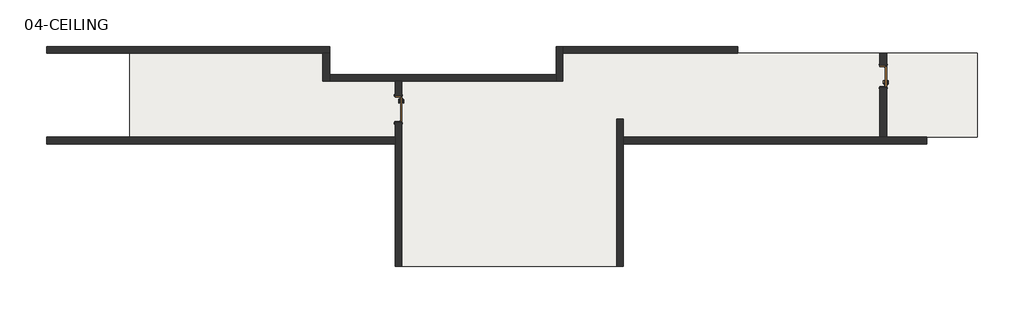
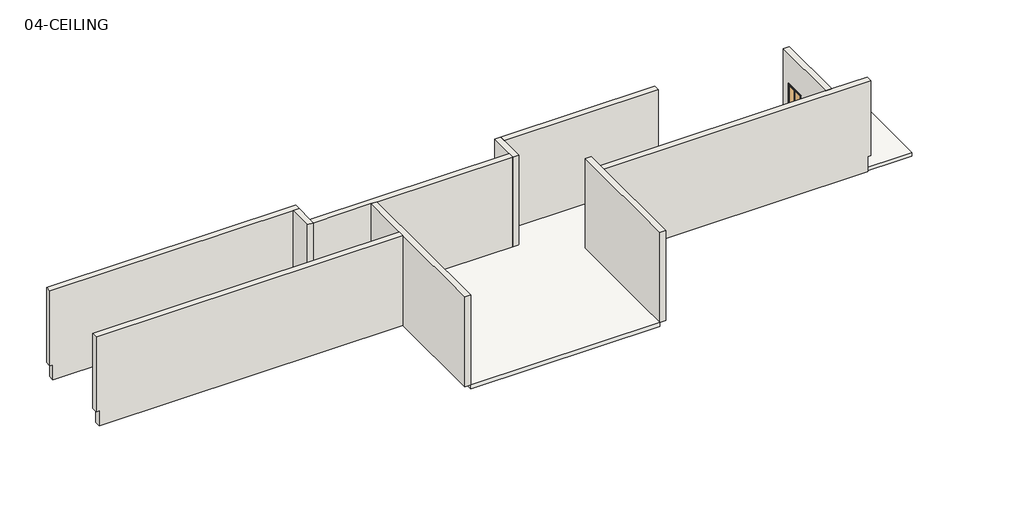
# One storey: 10 walls, 2 doors, 1 slab.
"""IFC4 building model written with IfcOpenShell, lengths in millimetres."""

from ifc_helpers import new_model, si_unit, frame, origin, place, context, project, spatial, polyline, outline, extrude, faceted_brep, transform, mapped, element, save
from components import doors_intsgl_d1_267d61ee, doors_intsgl_d2_251e2544

model = new_model("IFC4")

# Units and contexts
model_context = context("Model", 3, world=origin())
ifc_project = project(units=[si_unit("LENGTHUNIT", "METRE", prefix="MILLI")], contexts=[model_context])

# Site, building, storey
site = spatial("IfcSite", under=ifc_project)
building = spatial("IfcBuilding", under=site)
storey = spatial("IfcBuildingStorey", under=building, Name="04-CEILING", Elevation=3900.0)

# Doors
placement = place(None, origin())
doors_intsgl_d1_shape = doors_intsgl_d1_267d61ee(model_context)
element("IfcDoor", 1, ObjectType="Doors_IntSgl : D1", at=placement, inside=storey, context=model_context, shape_type="MappedRepresentation", body=[
    mapped(doors_intsgl_d1_shape, transform((2106.0830368, -5709.3092374, 3900.0), x_axis=(0.0, -1.0, 0.0), y_axis=(1.0, 0.0, 0.0), z_axis=(0.0, 0.0, 1.0))),
])
doors_intsgl_d2_shape = doors_intsgl_d2_251e2544(model_context)
element("IfcDoor", 2, ObjectType="Doors_IntSgl : D2", at=placement, inside=storey, context=model_context, shape_type="MappedRepresentation", body=[
    mapped(doors_intsgl_d2_shape, transform((18241.0830368, -4615.5592374, 3900.0), x_axis=(0.0, 1.0, 0.0), y_axis=(-1.0, 0.0, 0.0), z_axis=(0.0, 0.0, 1.0))),
])

# Slab
element("IfcSlab", 3, ObjectType="01-150 floor", at=placement, inside=storey, context=model_context, shape_type="SweptSolid", body=[
    extrude(outline(polyline([(-406.4169632, -3840.5592374), (-406.4169632, -4778.0592374), (7581.0830368, -4778.0592374), (7581.0830368, -3840.5592374), (21381.0830368, -3840.5592374), (21381.0830368, -6640.5592374), (9368.5830368, -6640.5592374), (9368.5830368, -10940.5592374), (2218.5830368, -10940.5592374), (2218.5830368, -6640.5592374), (-6843.9169632, -6640.5592374), (-6843.9169632, -3840.5592374), (-406.4169632, -3840.5592374)])), frame((0.0, 0.0, 3750.0), z_axis=(0.0, 0.0, 1.0), x_axis=(1.0, 0.0, 0.0)), (0.0, 0.0, 1.0), 150.0),
])

# Walls
element("IfcWall", 4, ObjectType="01-225 WALL", at=placement, inside=storey, context=model_context, shape_type="Brep", body=[
    faceted_brep([(-9493.9169632, -3840.5592374, 3900.0), (-406.4169632, -3840.5592374, 3900.0), (-181.4169632, -3840.5592374, 3900.0), (-181.4169632, -3840.5592374, 7500.0), (-406.4169632, -3840.5592374, 7500.0), (-9606.4169632, -3840.5592374, 7500.0), (-9606.4169632, -3840.5592374, 4500.0), (-9493.9169632, -3840.5592374, 4500.0), (-9493.9169632, -3615.5592374, 3900.0), (-9493.9169632, -3615.5592374, 4500.0), (-9606.4169632, -3615.5592374, 4500.0), (-9606.4169632, -3615.5592374, 7500.0), (-181.4169632, -3615.5592374, 7500.0), (-181.4169632, -3615.5592374, 3900.0), (-406.4169632, -3615.5592374, 3900.0)], [[[0, 1, 2, 3, 4, 5, 6, 7]], [[8, 9, 10, 11, 12, 13, 14]], [[2, 1, 0, 8, 14, 13]], [[5, 4, 3, 12, 11]], [[6, 5, 11, 10]], [[6, 10, 9, 7]], [[0, 7, 9, 8]], [[3, 2, 13, 12]]]),
])
element("IfcWall", 5, ObjectType="01-225 WALL", at=placement, inside=storey, context=model_context, shape_type="Brep", body=[
    faceted_brep([(-406.4169632, -3840.5592374, 3900.0), (-406.4169632, -4778.0592374, 3900.0), (-406.4169632, -4778.0592374, 7500.0), (-406.4169632, -3840.5592374, 7500.0), (-181.4169632, -3840.5592374, 3900.0), (-181.4169632, -3840.5592374, 7500.0), (-181.4169632, -4553.0592374, 7500.0), (-181.4169632, -4778.0592374, 7500.0), (-181.4169632, -4778.0592374, 3900.0), (-181.4169632, -4553.0592374, 3900.0)], [[[0, 1, 2, 3]], [[4, 5, 6, 7, 8, 9]], [[1, 0, 4, 9, 8]], [[3, 2, 7, 6, 5]], [[0, 3, 5, 4]], [[2, 1, 8, 7]]]),
])
element("IfcWall", 6, ObjectType="01-225 WALL", at=placement, inside=storey, context=model_context, shape_type="Brep", body=[
    faceted_brep([(7581.0830368, -4778.0592374, 3900.0), (7581.0830368, -3840.5592374, 3900.0), (7581.0830368, -3615.5592374, 3900.0), (7581.0830368, -3615.5592374, 7500.0), (7581.0830368, -3840.5592374, 7500.0), (7581.0830368, -4778.0592374, 7500.0), (7356.0830368, -4778.0592374, 3900.0), (7356.0830368, -4778.0592374, 7500.0), (7356.0830368, -4553.0592374, 7500.0), (7356.0830368, -3615.5592374, 7500.0), (7356.0830368, -3615.5592374, 3900.0), (7356.0830368, -4553.0592374, 3900.0)], [[[0, 1, 2, 3, 4, 5]], [[6, 7, 8, 9, 10, 11]], [[2, 1, 0, 6, 11, 10]], [[5, 4, 3, 9, 8, 7]], [[3, 2, 10, 9]], [[0, 5, 7, 6]]]),
])
element("IfcWall", 7, ObjectType="01-225 WALL", at=placement, inside=storey, context=model_context, shape_type="SweptSolid", body=[
    extrude(outline(polyline([(13406.0415807, -3840.5592374), (7581.0830368, -3840.5592374), (7581.0830368, -3615.5592374), (13406.0415807, -3615.5592374), (13406.0415807, -3840.5592374)])), frame((0.0, 0.0, 3900.0), z_axis=(0.0, 0.0, 1.0), x_axis=(1.0, 0.0, 0.0)), (0.0, 0.0, 1.0), 3600.0),
])
element("IfcWall", 8, ObjectType="01-225 WALL", at=placement, inside=storey, context=model_context, shape_type="Brep", body=[
    faceted_brep([(-181.4169632, -4778.0592374, 3900.0), (1993.5830368, -4778.0592374, 3900.0), (2218.5830368, -4778.0592374, 3900.0), (7356.0830368, -4778.0592374, 3900.0), (7356.0830368, -4778.0592374, 7500.0), (2218.5830368, -4778.0592374, 7500.0), (1993.5830368, -4778.0592374, 7500.0), (-181.4169632, -4778.0592374, 7500.0), (-181.4169632, -4553.0592374, 3900.0), (-181.4169632, -4553.0592374, 7500.0), (7356.0830368, -4553.0592374, 7500.0), (7356.0830368, -4553.0592374, 3900.0)], [[[0, 1, 2, 3, 4, 5, 6, 7]], [[8, 9, 10, 11]], [[3, 2, 1, 0, 8, 11]], [[7, 6, 5, 4, 10, 9]], [[4, 3, 11, 10]], [[0, 7, 9, 8]]]),
])
element("IfcWall", 9, ObjectType="01-225 WALL", at=placement, inside=storey, context=model_context, shape_type="SweptSolid", body=[
    extrude(outline(polyline([(3900.0, -9493.9169632), (3900.0, 1993.5830368), (7500.0, 1993.5830368), (7500.0, -9606.4169632), (4500.0, -9606.4169632), (4500.0, -9493.9169632), (3900.0, -9493.9169632)])), frame((0.0, -6865.5592374, 0.0), z_axis=(0.0, 1.0, 0.0), x_axis=(0.0, 0.0, 1.0)), (0.0, 0.0, 1.0), 225.0),
])
element("IfcWall", 10, ObjectType="01-225 WALL", at=placement, inside=storey, context=model_context, shape_type="Brep", body=[
    faceted_brep([(1993.5830368, -10940.5592374, 7500.0), (1993.5830368, -6865.5592374, 7500.0), (1993.5830368, -6640.5592374, 7500.0), (1993.5830368, -4778.0592374, 7500.0), (1993.5830368, -4778.0592374, 3900.0), (1993.5830368, -5259.3092374, 3900.0), (1993.5830368, -5259.3092374, 6300.0), (1993.5830368, -6159.3092374, 6300.0), (1993.5830368, -6159.3092374, 3900.0), (1993.5830368, -6640.5592374, 3900.0), (1993.5830368, -6865.5592374, 3900.0), (1993.5830368, -10940.5592374, 3900.0), (1993.5830368, -10940.5592374, 4500.0), (2218.5830368, -4778.0592374, 7500.0), (2218.5830368, -10940.5592374, 7500.0), (2218.5830368, -10940.5592374, 3900.0), (2218.5830368, -6159.3092374, 3900.0), (2218.5830368, -6159.3092374, 6300.0), (2218.5830368, -5259.3092374, 6300.0), (2218.5830368, -5259.3092374, 3900.0), (2218.5830368, -4778.0592374, 3900.0)], [[[0, 1, 2, 3, 4, 5, 6, 7, 8, 9, 10, 11, 12]], [[13, 14, 15, 16, 17, 18, 19, 20]], [[4, 20, 19, 5]], [[15, 11, 10, 9, 8, 16]], [[3, 2, 1, 0, 14, 13]], [[4, 3, 13, 20]], [[7, 17, 16, 8]], [[17, 7, 6, 18]], [[18, 6, 5, 19]], [[0, 12, 11, 15, 14]]]),
])
element("IfcWall", 11, ObjectType="01-225 WALL", at=placement, inside=storey, context=model_context, shape_type="Brep", body=[
    faceted_brep([(9593.5830368, -10940.5592374, 3900.0), (9593.5830368, -6865.5592374, 3900.0), (9593.5830368, -6640.5592374, 3900.0), (9593.5830368, -6040.5592374, 3900.0), (9593.5830368, -6040.5592374, 7500.0), (9593.5830368, -6640.5592374, 7500.0), (9593.5830368, -6865.5592374, 7500.0), (9593.5830368, -10940.5592374, 7500.0), (9593.5830368, -10940.5592374, 4500.0), (9368.5830368, -10940.5592374, 3900.0), (9368.5830368, -10940.5592374, 7500.0), (9368.5830368, -6040.5592374, 7500.0), (9368.5830368, -6040.5592374, 3900.0)], [[[0, 1, 2, 3, 4, 5, 6, 7, 8]], [[9, 10, 11, 12]], [[3, 2, 1, 0, 9, 12]], [[4, 3, 12, 11]], [[7, 6, 5, 4, 11, 10]], [[0, 8, 7, 10, 9]]]),
])
element("IfcWall", 12, ObjectType="01-225 WALL", at=placement, inside=storey, context=model_context, shape_type="Brep", body=[
    faceted_brep([(9593.5830368, -6865.5592374, 3900.0), (19581.0830368, -6865.5592374, 3900.0), (19581.0830368, -6865.5592374, 4500.0), (19693.5830368, -6865.5592374, 4500.0), (19693.5830368, -6865.5592374, 7500.0), (9593.5830368, -6865.5592374, 7500.0), (9593.5830368, -6640.5592374, 3900.0), (9593.5830368, -6640.5592374, 7500.0), (18128.5830368, -6640.5592374, 7500.0), (18353.5830368, -6640.5592374, 7500.0), (19693.5830368, -6640.5592374, 7500.0), (19693.5830368, -6640.5592374, 4500.0), (19581.0830368, -6640.5592374, 4500.0), (19581.0830368, -6640.5592374, 3900.0), (18353.5830368, -6640.5592374, 3900.0), (18128.5830368, -6640.5592374, 3900.0)], [[[0, 1, 2, 3, 4, 5]], [[6, 7, 8, 9, 10, 11, 12, 13, 14, 15]], [[1, 0, 6, 15, 14, 13]], [[5, 4, 10, 9, 8, 7]], [[0, 5, 7, 6]], [[4, 3, 11, 10]], [[11, 3, 2, 12]], [[2, 1, 13, 12]]]),
])
element("IfcWall", 13, ObjectType="01-225 WALL", at=placement, inside=storey, context=model_context, shape_type="SweptSolid", body=[
    extrude(outline(polyline([(-6640.5592374, 7500.0), (-3840.5592374, 7500.0), (-3840.5592374, 3900.0), (-4240.5592374, 3900.0), (-4240.5592374, 6300.0), (-4990.5592374, 6300.0), (-4990.5592374, 3900.0), (-6640.5592374, 3900.0), (-6640.5592374, 7500.0)])), frame((18128.5830368, 0.0, 0.0), z_axis=(1.0, 0.0, 0.0), x_axis=(0.0, 1.0, 0.0)), (0.0, 0.0, 1.0), 225.0),
])

save(model, "model.ifc")

# Revit data of these elements
# Type "Doors_IntSgl : D1"
#   Type Mark = "51"
#   Type Comments = "Internal Single"
#   Operation = "SingleSwingRight"
#   Manufacturer = "Revit"
#   Keynote = "L20"
#   Description = "Internal Single Door"
#   Analytic Construction = "Metal"
#   UnderCut = 8 mm
#   Tolerance = 2 mm
#   Thickness = 38 mm
#   Thermal Resistance (R) = 0.270117 (m²·K)/W
#   Structural Tolerance = 8 mm
#   StopDepth = 32 mm
#   Stop Thickness = 19 mm
#   Rough Width = 900 mm
#   Rough Height = 2400 mm
#   Height to Top Lock Rail = 1000 mm
#   Heat Transfer Coefficient (U) = 3.7021 W/(m²·K)
#   Handle Z Distance = 900 mm
#   Handle X Distance = 75 mm
#   Frame Thickness = 32 mm
#   Door Panel Width = 816 mm
#   Door Panel Thickness = 38 mm
#   Door Panel Offset = 0 mm
#   Height = 2400 mm
#   Width = 900 mm
#   Door Panel Height = 2350 mm
#   Architrave Setback = 5 mm
#   Vis - Ironmongery = yes
#   Define Thermal Properties by = 1
#   Material Ironmongery = Door - Handle
#   Material Frame = Door - Frame/Mullion (1)
#   Material Door = Door - Panel
#   Material Architrave = Door - Architrave
#   Visual Light Transmittance = 0
#   Solar Heat Gain Coefficient = 0
#   Function = (empty or 0)
#   Wall Closure = (empty or 0)
# Type "Doors_IntSgl : D2"
#   Type Mark = "52"
#   Type Comments = "Internal Single"
#   Operation = "SingleSwingRight"
#   Manufacturer = "Revit"
#   Keynote = "L20"
#   Description = "Internal Single Door"
#   Analytic Construction = "Metal"
#   UnderCut = 8 mm
#   Tolerance = 2 mm
#   Thickness = 38 mm
#   Thermal Resistance (R) = 0.270117 (m²·K)/W
#   Structural Tolerance = 8 mm
#   StopDepth = 32 mm
#   Stop Thickness = 19 mm
#   Rough Width = 750 mm
#   Rough Height = 2400 mm
#   Height to Top Lock Rail = 1000 mm
#   Heat Transfer Coefficient (U) = 3.7021 W/(m²·K)
#   Handle Z Distance = 900 mm
#   Handle X Distance = 75 mm
#   Frame Thickness = 32 mm
#   Door Panel Width = 666 mm
#   Door Panel Thickness = 38 mm
#   Door Panel Offset = 0 mm
#   Height = 2400 mm
#   Width = 750 mm
#   Door Panel Height = 2350 mm
#   Architrave Setback = 5 mm
#   Vis - Ironmongery = yes
#   Define Thermal Properties by = 1
#   Material Ironmongery = Door - Handle
#   Material Frame = Door - Frame/Mullion (1)
#   Material Door = Door - Panel
#   Material Architrave = Door - Architrave
#   Visual Light Transmittance = 0
#   Solar Heat Gain Coefficient = 0
#   Function = (empty or 0)
#   Wall Closure = (empty or 0)
# Type "01-150 floor"
#   Description = "Generic Floor (Material By Category), 12\" thick"
#   Assembly Code = "B1010"
#   Type Mark = "G01"
#   Function = 0
#   Layers, outside or top first: 150 mm no material (function 1)
# Type "01-225 WALL"
#   Description = "Generic Wall (Material By Category), 200mm thick"
#   Assembly Code = "B2010"
#   Type Mark = "G06"
#   Layers, outside or top first: 225 mm "01-WHITE WALL" (function 1)
# Element 1 (IfcDoor, "Doors_IntSgl : D1")
#   Phase Created = New Construction
#   Materials on its faces: "Door - Architrave", "Door - Handle", "Door - Frame/Mullion (1)", "Door - Panel"
# Element 2 (IfcDoor, "Doors_IntSgl : D2")
#   Phase Created = New Construction
#   Materials on its faces: "Door - Architrave", "Door - Handle", "Door - Frame/Mullion (1)", "Door - Panel"
# Element 3 (IfcSlab, "01-150 floor")
#   Height Offset From Level = 0 mm
#   Phase Created = New Construction
#   Materials on its faces: "Default Floor"
# Elements 4, 5, 6, 7, 8, 9, 10, 11, 12, 13 (IfcWall, "01-225 WALL")
#   Top Offset = 0 mm
#   Base Offset = 0 mm
#   wall height = 3600 mm
#   Phase Created = New Construction
#   Base Constraint = 04-CEILING
#   Materials on its faces: "01-WHITE WALL"
# Materials
#   "Door - Handle": colour RGB 0 0 0, transparency 0, Keynote = "P21", Cost = 0
#   "Door - Frame/Mullion (1)": class "Wood", colour RGB 212 179 113, transparency 0, Keynote = "L20", Cost = 0
#   "Door - Panel": class "Wood", colour RGB 210 159 95, transparency 0, Keynote = "L20", Cost = 0
#   "Door - Architrave": class "Wood", colour RGB 154 90 5, transparency 0, Keynote = "P20", Cost = 0
#   "01-WHITE WALL": class "Generic", colour RGB 244 244 244, transparency 0, Description = "Acoustic Ceiling Tile 24 x 48", Cost = 0
#   "Default Floor": colour RGB 128 128 128, transparency 0, Cost = 0
